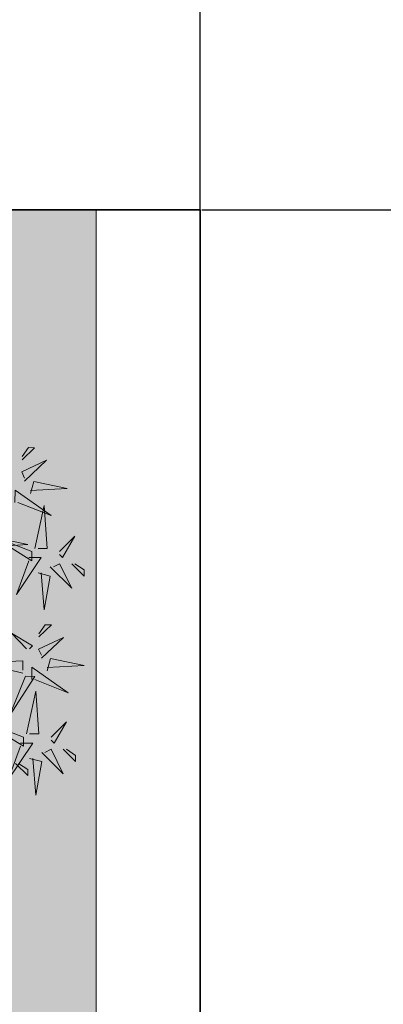
# Model space of a CAD drawing. Units: inches. Extents: x 1704 to 6393, y -157 to 1172.
# Tile 114 of 122: x 2716 to 2730, y 1003 to 1041. Entities that reach past the tile are written whole.
import ezdxf

# ---------------------------------------------------------------- set-up
doc = ezdxf.new("R2010")
doc.units = ezdxf.units.IN
doc.header["$MEASUREMENT"] = 0
for name, color, linetype, lineweight in [('A-ANNO-DIMS', 7, 'Continuous', 13), ('C-PROP', 7, 'Continuous', 35), ('L-HRDS', 8, 'Continuous', 18), ('L-shrub', 74, 'Continuous', 18)]:
    doc.layers.add(name, color=color, linetype=linetype, lineweight=lineweight)
doc.layers.add('L-HRDS-PATT', color=9, linetype='Continuous', lineweight=13, true_color=0xc5c1ba)
doc.styles.get("Standard").update_dxf_attribs({"font": 'arial.ttf'})
doc.dimstyles.get("Standard").update_dxf_attribs({"dimtxt": 6, "dimasz": 2, "dimexe": 0.18, "dimexo": 0.0625, "dimgap": 0.09, "dimtad": 0, "dimtih": 1, "dimtoh": 1, "dimdec": 1, "dimzin": 0, "dimdsep": 46, "dimlunit": 3, "dimtxsty": 'Standard', "dimblk": 'ARCHTICK', "dimcen": 0.09, "dimadec": 0, "dimazin": 0, "dimtfac": 1, "dimtdec": 1, "dimtofl": 0, "dimtmove": 0, "dimatfit": 3, "dimfxl": 1, "dimtolj": 1, "dimtzin": 0, "dimarcsym": 0})

# ---------------------------------------------------------------- blocks, each defined once
blk = doc.blocks.new('shrub3')
for points in [[(-263.24, 101.49), (-272.48, 103.79), (-267.86, 129.16), (-265.55, 101.49)], [(-272.48, 96.88), (-288.64, 113.02), (-279.4, 94.57), (-274.79, 96.88)], [(-256.32, 89.96), (-265.55, 89.96), (-247.08, 117.63), (-256.32, 92.27)], [(-252.6, 105.16), (-261.83, 114.38), (-261.83, 109.77), (-254.91, 105.16)], [(-288.64, 94.57), (-297.87, 103.79), (-297.87, 99.18), (-290.95, 94.57)], [(-279.4, 85.35), (-290.95, 73.82), (-281.71, 89.96), (-279.4, 87.65)], [(-258.63, 85.35), (-228.61, 73.82), (-258.63, 92.27), (-258.63, 85.35)], [(-260.93, 83.04), (-267.86, 50.76), (-270.17, 83.04), (-263.24, 83.04)], [(-260.26, 39.6), (-247.98, 69.31), (-267.17, 39.77), (-260.26, 39.6)], [(-264.81, 42.02), (-265.04, 32.79), (-292.24, 51.95), (-267.12, 42.08)], [(-258.01, 37.23), (-225.91, 29.5), (-258.24, 28), (-258.07, 34.92)], [(-276.51, 35.39), (-279.05, 26.21), (-304.29, 31.46), (-276.57, 33.08)], [(-272.13, 26.04), (-288.67, 10.29), (-270, 19.06), (-272.19, 23.73)], [(-260.78, 18.83), (-249.54, 7), (-265.45, 16.63), (-263.08, 18.88)], [(-270.23, 9.83), (-279.68, 0.83), (-275.07, 0.71), (-270.29, 7.52)], [(-269.6, -38.26), (-278.84, -35.95), (-274.22, -10.59), (-271.91, -38.26)], [(-262.68, -49.79), (-271.91, -49.79), (-253.44, -22.12), (-262.68, -47.48)], [(-278.84, -42.87), (-295, -26.73), (-285.76, -45.18), (-281.15, -42.87)], [(-295, -45.18), (-304.23, -35.95), (-304.23, -40.56), (-297.31, -45.18)], [(-285.76, -54.4), (-297.31, -65.93), (-288.07, -49.79), (-285.76, -52.09)], [(-264.99, -54.4), (-234.97, -65.93), (-264.99, -47.48), (-264.99, -54.4)], [(-267.29, -56.71), (-274.22, -88.99), (-276.53, -56.71), (-269.6, -56.71)], [(-234.11, -55.66), (-236.65, -64.84), (-261.89, -59.59), (-234.17, -57.97)], [(-252.09, -91.37), (-252.32, -100.61), (-279.52, -81.45), (-254.4, -91.32)], [(-263.79, -98.01), (-266.33, -107.18), (-291.57, -101.93), (-263.85, -100.32)], [(-259.41, -107.36), (-275.95, -123.11), (-257.28, -114.34), (-259.47, -109.66)], [(-257.51, -123.57), (-266.96, -132.57), (-262.35, -132.69), (-257.57, -125.88)]]:
    blk.add_lwpolyline(points)
blk = doc.blocks.new('_ArchTick')
at = {"color": 0, "linetype": 'ByBlock', "const_width": 0.15}
blk.add_lwpolyline([(-0.5, -0.5), (0.5, 0.5)], dxfattribs=at)
blk = doc.blocks.new('*D91')
at = {"layer": 'A-ANNO-DIMS', "color": 0, "lineweight": -2, "transparency": 16777216}
for p, q in [((2723.411, 1033.213), (2784.529, 1033.213)), ((2784.349, 1033.213), (2784.349, 517.868)), ((2784.349, -3.787), (2784.349, 511.557)), ((2723.411, -3.787), (2784.529, -3.787))]:
    blk.add_line(p, q, dxfattribs=at)
at = {"layer": 'Defpoints', "color": 0, "lineweight": -3, "transparency": 16777216}
for p in [(2723.349, 1033.213), (2784.349, 1033.213), (2723.349, -3.787)]:
    blk.add_point(p, dxfattribs=at)
at = {"layer": 'A-ANNO-DIMS', "color": 0, "lineweight": -2, "transparency": 16777216, "xscale": 2, "yscale": 2, "zscale": 2}
for p, rotation in [((2784.349, 1033.213), 90), ((2784.349, -3.787), 270)]:
    blk.add_blockref('_ArchTick', p, dxfattribs=dict(at, rotation=rotation))
at = {"layer": 'A-ANNO-DIMS', "color": 0, "transparency": 16777216, "insert": (2784.349, 514.713), "char_height": 6, "attachment_point": 5}
blk.add_mtext('\\A1;1037', dxfattribs=at)
blk = doc.blocks.new('*D95')
at = {"layer": 'A-ANNO-DIMS', "color": 0, "lineweight": -2, "transparency": 16777216}
for p, q in [((2605.349, 895.275), (2605.349, 1105.287)), ((2723.349, 895.275), (2723.349, 1105.287)), ((2605.349, 1105.107), (2657.907, 1105.107)), ((2723.349, 1105.107), (2670.791, 1105.107))]:
    blk.add_line(p, q, dxfattribs=at)
at = {"layer": 'Defpoints', "color": 0, "lineweight": -3, "transparency": 16777216}
for p in [(2723.349, 1105.107), (2605.349, 895.213), (2723.349, 895.213)]:
    blk.add_point(p, dxfattribs=at)
at = {"layer": 'A-ANNO-DIMS', "color": 0, "lineweight": -2, "transparency": 16777216, "xscale": 2, "yscale": 2, "zscale": 2, "rotation": 180}
blk.add_blockref('_ArchTick', (2605.349, 1105.107), dxfattribs=at)
at = {"layer": 'A-ANNO-DIMS', "color": 0, "lineweight": -2, "transparency": 16777216, "xscale": 2, "yscale": 2, "zscale": 2}
blk.add_blockref('_ArchTick', (2723.349, 1105.107), dxfattribs=at)
at = {"layer": 'A-ANNO-DIMS', "color": 0, "transparency": 16777216, "insert": (2664.349, 1105.107), "char_height": 6, "attachment_point": 5}
blk.add_mtext('\\A1;118', dxfattribs=at)

msp = doc.modelspace()

# ---------------------------------------------------------------- hatches: boundary and pattern name
at = {"layer": 'L-HRDS-PATT', "transparency": 33554661}
h = msp.add_hatch(color=256, dxfattribs=at)
h.dxf.hatch_style = 1
h.paths.add_polyline_path([(2719.349, 1033.213), (2664.349, 1033.213), (2664.349, 895.213), (2719.349, 895.213)])
h.paths.add_polyline_path([(2719.349, 895.213), (2664.349, 895.213), (2605.349, 895.213), (2605.349, 872.213), (2719.349, 872.213)])
h.paths.add_polyline_path([(2719.349, 872.213), (2605.349, 872.213), (2605.349, 854.213), (2601.349, 854.213, -0.121066), (2618.034, 850.113), (2618.05, 850.14), (2619.349, 849.39), (2601.349, 818.213), (2605.349, 818.213), (2605.349, 794.213), (2605.349, 754.213), (2631.349, 754.213), (2631.349, 716.213), (2719.349, 716.213)])

# ---------------------------------------------------------------- linework, layer by layer
at = {"layer": 'C-PROP'}
for p, q in [((2723.349, 1033.213), (1898.349, 1033.213)), ((2723.349, -3.787), (2723.349, 1033.213))]:
    msp.add_line(p, q, dxfattribs=at)
at = {"layer": 'L-HRDS'}
msp.add_line((2719.349, 5.658), (2719.349, 1033.213), dxfattribs=at)

# ---------------------------------------------------------------- block references
at = {"layer": 'L-shrub', "xscale": 0.0510581485411622, "yscale": 0.0510581485411622, "zscale": 0.0510581485411622, "rotation": 180}
msp.add_blockref('shrub3', (2703.343, 1017.291), dxfattribs=at)

# ---------------------------------------------------------------- dimensions: what is measured, and where the dimension line sits
at = {"layer": 'A-ANNO-DIMS'}
dim = msp.add_linear_dim(base=(2723.349, 1105.107), p1=(2605.349, 895.213), p2=(2723.349, 895.213), dimstyle='Standard', override={"dimdec": 0, "dimlfac": 1, "dimrnd": 0, "dimzin": 0, "dimdsep": 46, "dimlunit": 2}, dxfattribs=at)
dim.commit()
dim.dimension.update_dxf_attribs({"geometry": '*D95', "text_midpoint": (2664.349, 1105.107)})
dim = msp.add_linear_dim(base=(2784.349, 1033.213), p1=(2723.349, -3.787), p2=(2723.349, 1033.213), angle=90, dimstyle='Standard', override={"dimdec": 0, "dimlfac": 1, "dimrnd": 0, "dimzin": 0, "dimdsep": 46, "dimlunit": 2}, dxfattribs=at)
dim.commit()
dim.dimension.update_dxf_attribs({"geometry": '*D91', "text_midpoint": (2784.349, 514.713)})

doc.saveas('drawing.dxf')
